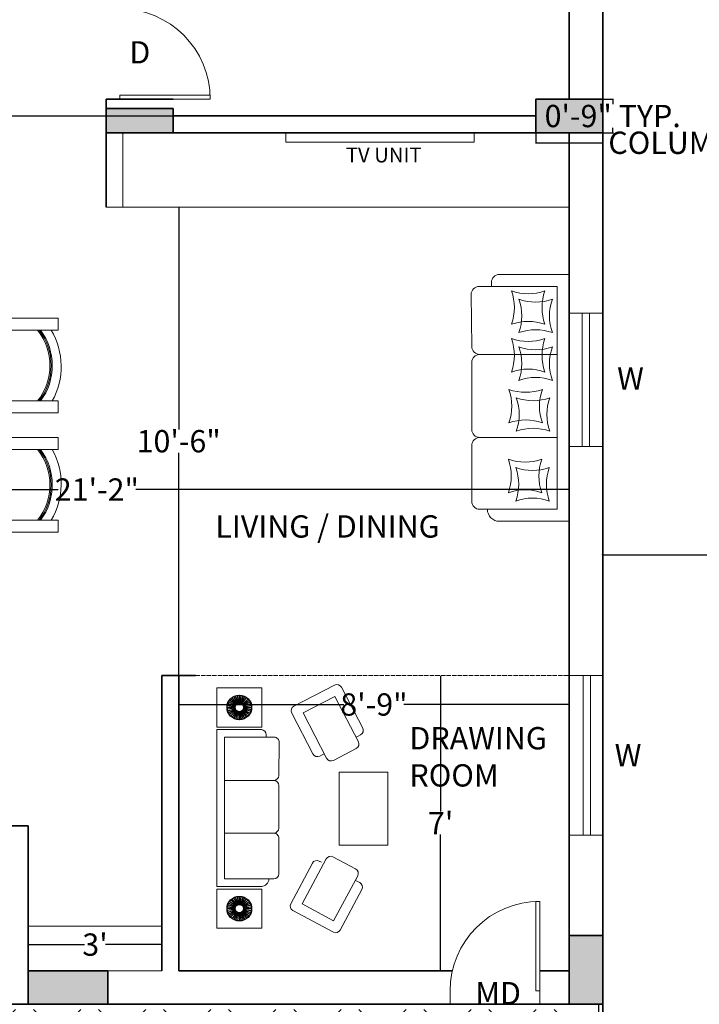
# Model space of a CAD drawing. Units: inches. Extents: x -2181 to 1225, y -80 to 4016.
# Tile 8 of 10: x 839 to 1021, y 191 to 456. Entities that reach past the tile are written whole.
import ezdxf

# ---------------------------------------------------------------- set-up
doc = ezdxf.new("R2010")
doc.units = ezdxf.units.IN
doc.header["$MEASUREMENT"] = 0
doc.linetypes.add('ACAD_ISO02W100', pattern=[15, 12, -3])
for name, color, linetype, lineweight in [('A-ANNO-DIMS', 2, 'Continuous', 18), ('A-ANNO-TEXT', 7, 'Continuous', 18), ('A-AREA-IDEN', 7, 'Continuous', 18), ('A-COLS', 7, 'Continuous', 35), ('A-COLS-PATT', 252, 'Continuous', 13), ('A-DOOR', 3, 'Continuous', 18), ('A-FLOR', 7, 'Continuous', 25), ('A-FLOR-PATT', 252, 'Continuous', 13), ('A-FURN', 30, 'Continuous', 18), ('A-GLAZ', 4, 'Continuous', 18), ('A-MILL', 8, 'Continuous', 18), ('A-WALL', 7, 'Continuous', 35), ('A-WALL-OVHD', 7, 'ACAD_ISO02W100', 18)]:
    doc.layers.add(name, color=color, linetype=linetype, lineweight=lineweight)
doc.layers.add('LAMP', color=2, linetype='Continuous')
doc.styles.get("Standard").update_dxf_attribs({"font": 'arial.ttf'})
doc.dimstyles.get("Standard").update_dxf_attribs({"dimtxt": 6, "dimasz": 0.18, "dimexe": 0.18, "dimexo": 0.0625, "dimgap": 0.09, "dimtad": 0, "dimtih": 1, "dimtoh": 1, "dimdec": 4, "dimzin": 0, "dimdsep": 46, "dimlunit": 4, "dimtxsty": 'Standard', "dimcen": 0.09, "dimadec": 0, "dimazin": 0, "dimtfac": 1, "dimtdec": 4, "dimtofl": 0, "dimtmove": 0, "dimatfit": 3, "dimfxl": 1, "dimtolj": 1, "dimtzin": 0, "dimarcsym": 0})

# ---------------------------------------------------------------- blocks, each defined once
blk = doc.blocks.new('*U2')
for p, q in [((0, 0), (0, -6)), ((40, 0), (40, -6))]:
    blk.add_line(p, q)
blk.add_lwpolyline([(0, 0), (0, 40), (1.75, 40), (1.75, 0)], close=True)
blk.add_arc((0, 0), 40, 0, 90)
blk = doc.blocks.new('*U18')
blk.add_line((3.3, 4.46), (3.3, 6.59))
for radius in [3.3, 1.16]:
    blk.add_circle((3.3, 3.3), radius)
blk = doc.blocks.new('*U17')
at = {"layer": 'LAMP', "transparency": 16777216}
for p, rotation in [((-44.82, 106.18), 44.99999999999992), ((-40.16, 110.84), 134.9999999999996), ((-44.82, 115.5), 224.9999999999994), ((-49.48, 110.84), 314.9999999999993), ((-45.55, 106.23), 35.99999999999994), ((-44.09, 106.23), 53.9999999999999), ((-40.22, 110.11), 125.9999999999997), ((-40.22, 111.57), 143.9999999999996), ((-44.09, 115.44), 215.9999999999994), ((-45.55, 115.44), 233.9999999999994), ((-49.43, 111.57), 305.9999999999992), ((-49.43, 110.11), 323.9999999999993), ((-46.26, 106.4), 26.99999999999998), ((-43.38, 106.4), 62.99999999999984), ((-40.39, 109.4), 116.9999999999997), ((-40.39, 112.28), 152.9999999999996), ((-43.38, 115.27), 206.9999999999994), ((-46.26, 115.27), 242.9999999999994), ((-49.26, 112.28), 296.9999999999993), ((-49.26, 109.4), 332.9999999999992), ((-46.94, 106.68), 17.99999999999997), ((-42.7, 106.68), 71.9999999999998), ((-40.67, 108.72), 107.9999999999997), ((-40.67, 112.96), 161.9999999999995), ((-42.7, 114.99), 197.9999999999995), ((-46.94, 114.99), 251.9999999999995), ((-48.98, 112.96), 287.9999999999994), ((-48.98, 108.72), 341.9999999999992), ((-47.56, 107.07), 8.999999999999984), ((-42.08, 107.07), 80.99999999999979), ((-41.05, 108.1), 98.99999999999974), ((-41.05, 113.58), 170.9999999999995), ((-42.08, 114.61), 188.9999999999995), ((-47.56, 114.61), 260.9999999999993), ((-48.59, 113.58), 278.9999999999992), ((-48.59, 108.1), 350.9999999999993), ((-41.52, 107.54), 89.99999999999976), ((-41.52, 114.14), 180), ((-48.12, 114.14), 269.9999999999993)]:
    blk.add_blockref('*U18', p, dxfattribs=dict(at, rotation=rotation))
blk.add_blockref('*U18', (-48.12, 107.54), dxfattribs=at)
blk = doc.blocks.new('*U15')
blk.add_line((3.3, 4.46), (3.3, 6.59))
for radius in [3.3, 1.16]:
    blk.add_circle((3.3, 3.3), radius)
blk = doc.blocks.new('*U16')
at = {"layer": 'LAMP', "transparency": 16777216}
for p, rotation in [((-44.82, 106.18), 44.99999999999992), ((-40.16, 110.84), 134.9999999999996), ((-44.82, 115.5), 224.9999999999994), ((-49.48, 110.84), 314.9999999999993), ((-45.55, 106.23), 35.99999999999994), ((-44.09, 106.23), 53.9999999999999), ((-40.22, 110.11), 125.9999999999997), ((-40.22, 111.57), 143.9999999999996), ((-44.09, 115.44), 215.9999999999994), ((-45.55, 115.44), 233.9999999999994), ((-49.43, 111.57), 305.9999999999992), ((-49.43, 110.11), 323.9999999999993), ((-46.26, 106.4), 26.99999999999998), ((-43.38, 106.4), 62.99999999999984), ((-40.39, 109.4), 116.9999999999997), ((-40.39, 112.28), 152.9999999999996), ((-43.38, 115.27), 206.9999999999994), ((-46.26, 115.27), 242.9999999999994), ((-49.26, 112.28), 296.9999999999993), ((-49.26, 109.4), 332.9999999999992), ((-46.94, 106.68), 17.99999999999997), ((-42.7, 106.68), 71.9999999999998), ((-40.67, 108.72), 107.9999999999997), ((-40.67, 112.96), 161.9999999999995), ((-42.7, 114.99), 197.9999999999995), ((-46.94, 114.99), 251.9999999999995), ((-48.98, 112.96), 287.9999999999994), ((-48.98, 108.72), 341.9999999999992), ((-47.56, 107.07), 8.999999999999984), ((-42.08, 107.07), 80.99999999999979), ((-41.05, 108.1), 98.99999999999974), ((-41.05, 113.58), 170.9999999999995), ((-42.08, 114.61), 188.9999999999995), ((-47.56, 114.61), 260.9999999999993), ((-48.59, 113.58), 278.9999999999992), ((-48.59, 108.1), 350.9999999999993), ((-41.52, 107.54), 89.99999999999976), ((-41.52, 114.14), 180), ((-48.12, 114.14), 269.9999999999993)]:
    blk.add_blockref('*U15', p, dxfattribs=dict(at, rotation=rotation))
blk.add_blockref('*U15', (-48.12, 107.54), dxfattribs=at)
blk = doc.blocks.new('*D25')
at = {"layer": 'A-ANNO-DIMS', "color": 0, "lineweight": -2, "transparency": 16777216}
for p, q in [((995.51, 312.49), (995.51, 312.61)), ((1087.01, 312.49), (1087.01, 312.61)), ((995.69, 312.43), (1031.04, 312.43)), ((1086.83, 312.43), (1051.49, 312.43))]:
    blk.add_line(p, q, dxfattribs=at)
at = {"layer": 'A-ANNO-DIMS', "color": 0, "transparency": 16777216}
for points in [[(995.69, 312.46), (995.69, 312.4), (995.51, 312.43)], [(1086.83, 312.46), (1086.83, 312.4), (1087.01, 312.43)]]:
    blk.add_solid(points, dxfattribs=at)
at = {"layer": 'Defpoints', "color": 0, "transparency": 16777216}
for p in [(995.51, 312.43), (1087.01, 312.43), (1087.01, 312.43)]:
    blk.add_point(p, dxfattribs=at)
at = {"layer": 'A-ANNO-DIMS', "color": 0, "transparency": 16777216, "insert": (1041.26, 312.43), "char_height": 6, "attachment_point": 5}
blk.add_mtext('\\A1;7\'-7{\\H1x;\\S1/2;}"', dxfattribs=at)
blk = doc.blocks.new('*D53')
at = {"layer": 'A-ANNO-DIMS', "color": 0, "lineweight": -2, "transparency": 16777216}
for p, q in [((881.51, 279.92), (881.51, 271.97)), ((986.51, 279.92), (986.51, 271.97)), ((881.69, 272.15), (925.95, 272.15)), ((986.33, 272.15), (942.08, 272.15))]:
    blk.add_line(p, q, dxfattribs=at)
at = {"layer": 'A-ANNO-DIMS', "color": 0, "transparency": 16777216}
for points in [[(881.69, 272.18), (881.69, 272.12), (881.51, 272.15)], [(986.33, 272.18), (986.33, 272.12), (986.51, 272.15)]]:
    blk.add_solid(points, dxfattribs=at)
at = {"layer": 'Defpoints', "color": 0, "transparency": 16777216}
for p in [(881.51, 279.98), (986.51, 279.98), (986.51, 272.15)]:
    blk.add_point(p, dxfattribs=at)
at = {"layer": 'A-ANNO-DIMS', "color": 0, "transparency": 16777216, "insert": (934.01, 272.15), "char_height": 6, "attachment_point": 5}
blk.add_mtext('\\A1;8\'-9"', dxfattribs=at)
blk = doc.blocks.new('*D54')
at = {"layer": 'A-ANNO-DIMS', "color": 0, "lineweight": -2, "transparency": 16777216}
for p, q in [((951.95, 279.8), (951.95, 243.32)), ((952.01, 279.98), (952.13, 279.98)), ((951.95, 200.66), (951.95, 237.14)), ((955.06, 200.48), (951.77, 200.48))]:
    blk.add_line(p, q, dxfattribs=at)
at = {"layer": 'A-ANNO-DIMS', "color": 0, "transparency": 16777216}
for points in [[(951.92, 279.8), (951.98, 279.8), (951.95, 279.98)], [(951.92, 200.66), (951.98, 200.66), (951.95, 200.48)]]:
    blk.add_solid(points, dxfattribs=at)
at = {"layer": 'Defpoints', "color": 0, "transparency": 16777216}
for p in [(951.95, 279.98), (951.95, 279.98), (955.12, 200.48)]:
    blk.add_point(p, dxfattribs=at)
at = {"layer": 'A-ANNO-DIMS', "color": 0, "transparency": 16777216, "insert": (951.95, 240.23), "char_height": 6, "attachment_point": 5}
blk.add_mtext("\\A1;7'", dxfattribs=at)
blk = doc.blocks.new('*D55')
at = {"layer": 'A-ANNO-DIMS', "color": 0, "lineweight": -2, "transparency": 16777216}
for p, q in [((841.01, 212.42), (841.01, 207.37)), ((877.01, 212.42), (877.01, 207.37)), ((841.19, 207.55), (856.17, 207.55)), ((876.83, 207.55), (861.86, 207.55))]:
    blk.add_line(p, q, dxfattribs=at)
at = {"layer": 'A-ANNO-DIMS', "color": 0, "transparency": 16777216}
for points in [[(841.19, 207.58), (841.19, 207.52), (841.01, 207.55)], [(876.83, 207.58), (876.83, 207.52), (877.01, 207.55)]]:
    blk.add_solid(points, dxfattribs=at)
at = {"layer": 'Defpoints', "color": 0, "transparency": 16777216}
for p in [(841.01, 212.48), (877.01, 212.48), (877.01, 207.55)]:
    blk.add_point(p, dxfattribs=at)
at = {"layer": 'A-ANNO-DIMS', "color": 0, "transparency": 16777216, "insert": (859.01, 207.55), "char_height": 6, "attachment_point": 5}
blk.add_mtext("\\A1;3'", dxfattribs=at)
blk = doc.blocks.new('*D57')
at = {"layer": 'A-ANNO-DIMS', "color": 0, "lineweight": -2, "transparency": 16777216}
for p, q in [((732.51, 330.05), (732.51, 330.16)), ((732.69, 329.98), (849.07, 329.98)), ((986.33, 329.98), (869.96, 329.98)), ((986.51, 330.05), (986.51, 330.16))]:
    blk.add_line(p, q, dxfattribs=at)
at = {"layer": 'A-ANNO-DIMS', "color": 0, "transparency": 16777216}
for points in [[(732.69, 330.01), (732.69, 329.95), (732.51, 329.98)], [(986.33, 330.01), (986.33, 329.95), (986.51, 329.98)]]:
    blk.add_solid(points, dxfattribs=at)
at = {"layer": 'Defpoints', "color": 0, "transparency": 16777216}
for p in [(732.51, 329.98), (986.51, 329.98), (986.51, 329.98)]:
    blk.add_point(p, dxfattribs=at)
at = {"layer": 'A-ANNO-DIMS', "color": 0, "transparency": 16777216, "insert": (859.51, 329.98), "char_height": 6, "attachment_point": 5}
blk.add_mtext('\\A1;21\'-2"', dxfattribs=at)
blk = doc.blocks.new('*D58')
at = {"layer": 'A-ANNO-DIMS', "color": 0, "lineweight": -2, "transparency": 16777216}
for p, q in [((881.51, 405.8), (881.51, 346.14)), ((881.58, 405.98), (881.69, 405.98)), ((881.51, 280.16), (881.51, 339.83)), ((881.58, 279.98), (881.69, 279.98))]:
    blk.add_line(p, q, dxfattribs=at)
at = {"layer": 'A-ANNO-DIMS', "color": 0, "transparency": 16777216}
for points in [[(881.48, 405.8), (881.54, 405.8), (881.51, 405.98)], [(881.48, 280.16), (881.54, 280.16), (881.51, 279.98)]]:
    blk.add_solid(points, dxfattribs=at)
at = {"layer": 'Defpoints', "color": 0, "transparency": 16777216}
for p in [(881.51, 405.98), (881.51, 405.98), (881.51, 279.98)]:
    blk.add_point(p, dxfattribs=at)
at = {"layer": 'A-ANNO-DIMS', "color": 0, "transparency": 16777216, "insert": (881.51, 342.98), "char_height": 6, "attachment_point": 5}
blk.add_mtext('\\A1;10\'-6"', dxfattribs=at)
blk = doc.blocks.new('DINING-CHAIR-SIDE')
for p, q in [((0.79, 22.26), (0.79, 25.47)), ((19.33, 22.26), (19.33, 25.47)), ((0.79, 0), (0.79, 3.21)), ((19.33, 3.21), (19.33, 0))]:
    blk.add_line(p, q)
for points in [[(0.79, 25.47), (19.33, 25.47)], [(0.79, 22.26), (22.53, 22.26), (22.53, 3.21), (0.79, 3.21)], [(19.33, 0), (0.79, 0)]]:
    blk.add_lwpolyline(points)
for centre, radius, start, end in [((19.12, 12.45), 19.13, 149.1418, 208.8973), ((18.29, 12.73), 15.92, 143.2428, 216.7572), ((18.29, 12.73), 15.6, 142.3578, 217.6422), ((18.29, 12.73), 15.28, 141.4242, 218.5758)]:
    blk.add_arc(centre, radius, start, end)
blk = doc.blocks.new('COL-18X9')
blk.add_lwpolyline([(0, 9), (18, 9), (18, 0), (0, 0)], close=True)
blk = doc.blocks.new('*D98')
at = {"layer": 'A-ANNO-DIMS', "color": 0, "lineweight": -2, "transparency": 16777216}
for p, q in [((977.51, 425.92), (977.51, 423.1)), ((995.51, 425.92), (995.51, 423.1)), ((977.69, 423.28), (995.33, 423.28)), ((995.51, 423.28), (995.69, 423.28))]:
    blk.add_line(p, q, dxfattribs=at)
at = {"layer": 'A-ANNO-DIMS', "color": 0, "transparency": 16777216}
for points in [[(977.69, 423.31), (977.69, 423.25), (977.51, 423.28)], [(995.33, 423.31), (995.33, 423.25), (995.51, 423.28)]]:
    blk.add_solid(points, dxfattribs=at)
at = {"layer": 'Defpoints', "color": 0, "transparency": 16777216}
for p in [(977.51, 425.98), (995.51, 425.98), (995.51, 423.28)]:
    blk.add_point(p, dxfattribs=at)
at = {"layer": 'A-ANNO-DIMS', "color": 0, "transparency": 16777216, "insert": (1033.36, 423.28), "char_height": 6, "attachment_point": 5}
blk.add_mtext('\\A1;COLUMN 1\'-6" TYP.', dxfattribs=at)
blk = doc.blocks.new('*D99')
at = {"layer": 'A-ANNO-DIMS', "color": 0, "lineweight": -2, "transparency": 16777216}
for p, q in [((995.58, 434.98), (998.39, 434.98)), ((998.21, 434.8), (998.21, 433.64)), ((998.21, 426.16), (998.21, 427.33)), ((995.58, 425.98), (998.39, 425.98))]:
    blk.add_line(p, q, dxfattribs=at)
at = {"layer": 'A-ANNO-DIMS', "color": 0, "transparency": 16777216}
for points in [[(998.18, 434.8), (998.24, 434.8), (998.21, 434.98)], [(998.18, 426.16), (998.24, 426.16), (998.21, 425.98)]]:
    blk.add_solid(points, dxfattribs=at)
at = {"layer": 'Defpoints', "color": 0, "transparency": 16777216}
for p in [(995.51, 434.98), (998.21, 434.98), (995.51, 425.98)]:
    blk.add_point(p, dxfattribs=at)
at = {"layer": 'A-ANNO-DIMS', "color": 0, "transparency": 16777216, "insert": (998.21, 430.48), "char_height": 6, "attachment_point": 5}
blk.add_mtext('\\A1;0\'-9" TYP.', dxfattribs=at)
blk = doc.blocks.new('*D131')
at = {"layer": 'A-ANNO-DIMS', "color": 0, "lineweight": -2, "transparency": 16777216}
for p, q in [((976.64, 563.98), (-59.44, 563.98)), ((-59.26, 563.8), (-59.26, 500.43)), ((-59.26, 430.66), (-59.26, 494.04)), ((977.45, 430.48), (-59.44, 430.48))]:
    blk.add_line(p, q, dxfattribs=at)
at = {"layer": 'A-ANNO-DIMS', "color": 0, "transparency": 16777216}
for points in [[(-59.29, 563.8), (-59.23, 563.8), (-59.26, 563.98)], [(-59.29, 430.66), (-59.23, 430.66), (-59.26, 430.48)]]:
    blk.add_solid(points, dxfattribs=at)
at = {"layer": 'Defpoints', "color": 0, "transparency": 16777216}
for p in [(976.7, 563.98), (-59.26, 430.48), (977.51, 430.48)]:
    blk.add_point(p, dxfattribs=at)
at = {"layer": 'A-ANNO-DIMS', "color": 0, "transparency": 16777216, "insert": (-59.26, 497.23), "char_height": 6, "attachment_point": 5}
blk.add_mtext('\\A1;11\'-1 1/2"', dxfattribs=at)

msp = doc.modelspace()

# ---------------------------------------------------------------- hatches: boundary and pattern name
at = {"layer": 'A-COLS-PATT'}
h = msp.add_hatch(color=256, dxfattribs=at)
h.dxf.hatch_style = 1
h.paths.add_polyline_path([(995.51461, 209.98479), (986.51461, 209.98479), (986.51461, 191.48479), (995.51461, 191.48479)])
h.paths.add_polyline_path([(862.50488, 191.48479), (862.50488, 200.48479), (841.01461, 200.48479), (841.01461, 191.48479)])
h.paths.add_polyline_path([(995.51461, 425.98479), (995.51461, 434.98479), (977.51461, 434.98479), (977.51461, 425.98479)])
h.paths.add_polyline_path([(880.01461, 425.98479), (880.01461, 432.54138), (862.01461, 432.54138), (862.01461, 425.98479)])
h.paths.add_polyline_path([(880.82546, 563.98479), (880.82546, 572.98479), (862.01461, 572.98479), (862.01461, 563.98479)])
h.paths.add_polyline_path([(995.51461, 563.98479), (995.51461, 572.98479), (976.70377, 572.98479), (976.70377, 563.98479)])
h.paths.add_polyline_path([(674.51461, 572.98479), (665.51461, 572.98479), (665.51461, 556.48479), (674.51461, 556.48479)])
h.paths.add_polyline_path([(674.51461, 442.48479), (665.51461, 442.48479), (665.51461, 425.98479), (674.51461, 425.98479)])
at = {"layer": 'A-FLOR-PATT'}
h = msp.add_hatch(dxfattribs=at)
h.set_pattern_fill('ANGLE', color=256, scale=45, angle=45)
h.set_pattern_definition([(45, (0, 0), (-8.75045, 8.75045), [9, -3.375]), (135, (0, 0), (-8.75045, -8.75045), [9, -3.375])])
h.paths.add_polyline_path([(665.51461, 191.48479), (665.51461, 136.48479), (674.51461, 136.48479), (674.51461, 137.48479), (994.51461, 137.48479), (994.51461, 191.48479)])

# ---------------------------------------------------------------- linework, layer by layer
at = {"layer": 'A-COLS'}
for p, q in [((977.51461, 434.98479), (995.51461, 434.98479)), ((880.01461, 432.54138), (862.01461, 432.54138)), ((986.51461, 425.98479), (995.51461, 425.98479))]:
    msp.add_line(p, q, dxfattribs=at)
for points in [[(880.01461, 432.54138), (880.01461, 425.98479), (862.01461, 425.98479), (862.01461, 434.98479), (880.01461, 434.98479)], [(977.51461, 425.98479), (977.51461, 434.98479)], [(986.51461, 209.98479), (995.51461, 209.98479)]]:
    msp.add_lwpolyline(points, dxfattribs=at)
msp.add_lwpolyline([(841.01461, 200.48479), (862.50488, 200.48479), (862.50488, 191.48479), (841.01461, 191.48479)], close=True, dxfattribs=at)
at = {"layer": 'A-FLOR'}
msp.add_lwpolyline([(994.51461, 137.48479), (994.51461, 191.48479)], dxfattribs=at)
at = {"layer": 'A-FURN'}
for p, q in [((983.28882, 366.34519), (962.47646, 366.34519)), ((961.4012, 344.01286), (961.4012, 344.01067)), ((983.28882, 344.00116), (962.4774, 344.01021)), ((920.66303, 258.90305), (919.75396, 258.42993)), ((893.8348, 251.72826), (907.05875, 251.72826)), ((893.8348, 237.5311), (907.05816, 237.53685)), ((907.74196, 237.53853), (907.74196, 237.53714))]:
    msp.add_line(p, q, dxfattribs=at)
for points in [[(986.51461, 321.4323), (986.51461, 387.85049), (967.75164, 387.85049, 0.414213562), (965.60111, 385.69996), (965.60111, 384.62469)], [(983.28882, 324.6581), (983.28882, 384.62469), (962.30166, 384.62469, 0.417877186), (960.1513, 382.4473), (960.32593, 368.46885, 0.410559405), (962.47629, 366.34519), (983.28882, 366.34519)], [(960.32593, 364.19466), (960.32593, 346.16339, 0.414213562), (962.47646, 344.01286), (983.28882, 344.01286)], [(960.32593, 341.85968), (960.32593, 326.80862, 0.414213562), (962.47646, 324.6581), (983.28882, 324.6581)], [(964.52584, 324.6581), (964.52584, 324.6581, 0.414213562), (967.75164, 321.4323), (986.51461, 321.4323)], [(920.05698, 258.58764), (919.45094, 258.27222, -0.414213562), (917.60802, 258.85348), (911.9007, 269.81962, -0.414213562), (912.48196, 271.66254), (923.43749, 277.36434, -0.414213562), (925.28041, 276.78308), (930.98773, 265.81695, -0.414213562), (930.40647, 263.97402), (929.80042, 263.65861), (929.19438, 263.34319)], [(891.78516, 223.19108), (891.78516, 265.3925), (903.70696, 265.3925, -0.414213562), (905.07338, 264.02608), (905.07338, 263.34287)], [(893.8348, 225.24072), (893.8348, 263.34287), (907.16982, 263.34287, -0.417877186), (908.53613, 261.95937), (908.42518, 253.07762, -0.410559405), (907.05886, 251.72826), (893.8348, 251.72826)], [(908.42518, 250.36184), (908.42518, 238.90496, -0.414213562), (907.05875, 237.53853), (893.8348, 237.53853)], [(908.42518, 236.17042), (908.42518, 226.60714, -0.414213562), (907.05875, 225.24072), (893.8348, 225.24072)], [(919.90911, 229.70718), (919.30633, 230.02879, 0.414213562), (917.45755, 229.46643), (911.63823, 218.55932, 0.414213562), (912.20059, 216.71054), (923.09715, 210.89685, 0.414213562), (924.94593, 211.4592), (930.76525, 222.36632, 0.414213562), (930.20289, 224.2151), (929.60011, 224.53671), (928.99733, 224.85831)], [(905.75659, 225.24072), (905.75659, 225.24072, -0.414213562), (903.70696, 223.19108), (891.78516, 223.19108)]]:
    msp.add_lwpolyline(points, format="xyb", dxfattribs=at)
for points in [[(967.75164, 387.85049), (967.51697, 387.85049)], [(967.51697, 321.4323), (967.75164, 321.4323)], [(891.78516, 276.64518), (891.78516, 266.07571)], [(903.85606, 276.64518), (891.78516, 276.64518)], [(891.78516, 276.64518), (891.78516, 266.07571)], [(903.85606, 276.64518), (891.78516, 276.64518)], [(903.85606, 266.07571), (903.85606, 276.64518)], [(903.85606, 266.07571), (903.85606, 276.64518)], [(891.78516, 266.07571), (903.85606, 266.07571)], [(891.78516, 266.07571), (903.85606, 266.07571)], [(903.70696, 265.3925), (903.85606, 265.3925)], [(903.85606, 223.19108), (903.70696, 223.19108)], [(891.78516, 222.50787), (891.78516, 211.93841)], [(903.85606, 222.50787), (891.78516, 222.50787)], [(891.78516, 222.50787), (891.78516, 211.93841)], [(903.85606, 222.50787), (891.78516, 222.50787)], [(891.78516, 222.50787), (891.78516, 211.93841)], [(903.85606, 222.50787), (891.78516, 222.50787)], [(903.85606, 211.93841), (903.85606, 222.50787)], [(903.85606, 211.93841), (903.85606, 222.50787)], [(903.85606, 211.93841), (903.85606, 222.50787)], [(891.78516, 211.93841), (903.85606, 211.93841)], [(891.78516, 211.93841), (903.85606, 211.93841)], [(891.78516, 211.93841), (903.85606, 211.93841)]]:
    msp.add_lwpolyline(points, dxfattribs=at)
for points in [[(921.29386, 257.69096), (914.95571, 269.86919), (923.48706, 274.30933), (929.82521, 262.1311, -0.414213562), (929.24395, 260.28817), (923.13679, 257.1097, -0.414213562)], [(921.1551, 230.59115), (914.69258, 218.47846), (923.17801, 213.9512), (929.64054, 226.06388, 0.414213562), (929.07818, 227.91266), (923.00388, 231.1535, 0.414213562)]]:
    msp.add_lwpolyline(points, format="xyb", close=True, dxfattribs=at)
msp.add_lwpolyline([(924.68117, 253.97634), (937.72776, 253.97634), (937.72776, 234.27037), (924.68117, 234.27037)], close=True, dxfattribs=at)
for centre, radius, start, end in [((975.48814, 395.98818), 13.32748, 250.2663432, 289.7336568), ((958.44335, 378.94339), 13.32748, 340.2663432, 19.7336568), ((992.53293, 378.94339), 13.32748, 160.2663432, 199.7336568), ((977.48811, 393.74472), 13.32748, 250.2663432, 289.7336568), ((960.44332, 376.69994), 13.32748, 340.2663432, 19.7336568), ((994.53289, 376.69994), 13.32748, 160.2663432, 199.7336568), ((975.48814, 361.8986), 13.32748, 70.2663432, 109.7336568), ((977.48811, 359.65515), 13.32748, 70.2663432, 109.7336568), ((975.48814, 383.14097), 13.32748, 250.2663432, 289.7336568), ((958.44335, 366.09619), 13.32748, 340.2663432, 19.7336568), ((977.48811, 380.89752), 13.32748, 250.2663432, 289.7336568), ((960.44332, 363.85273), 13.32748, 340.2663432, 19.7336568), ((992.53293, 366.09619), 13.32748, 160.2663432, 199.7336568), ((994.53289, 363.85273), 13.32748, 160.2663432, 199.7336568), ((962.47646, 364.19466), 2.15053, 90, 180), ((975.48814, 349.0514), 13.32748, 70.2663432, 109.7336568), ((977.48811, 346.80795), 13.32748, 70.2663432, 109.7336568), ((974.79693, 369.46492), 13.32748, 250.2663432, 289.7336568), ((957.75215, 352.42014), 13.32748, 340.2663432, 19.7336568), ((991.84172, 352.42014), 13.32748, 160.2663432, 199.7336568), ((976.7969, 367.22147), 13.32748, 250.2663432, 289.7336568), ((959.75211, 350.17668), 13.32748, 340.2663432, 19.7336568), ((993.84169, 350.17668), 13.32748, 160.2663432, 199.7336568), ((974.79693, 335.37535), 13.32748, 70.2663432, 109.7336568), ((976.7969, 333.1319), 13.32748, 70.2663432, 109.7336568), ((962.47646, 341.85968), 2.15053, 89.9751027, 180), ((974.65869, 350.67762), 13.32748, 250.2663432, 289.7336568), ((957.6139, 333.63283), 13.32748, 340.2663432, 19.7336568), ((991.70348, 333.63283), 13.32748, 160.2663432, 199.7336568), ((976.65866, 348.43417), 13.32748, 250.2663432, 289.7336568), ((959.61387, 331.38938), 13.32748, 340.2663432, 19.7336568), ((993.70345, 331.38938), 13.32748, 160.2663432, 199.7336568), ((974.65869, 316.58805), 13.32748, 70.2663432, 109.7336568), ((976.65866, 314.34459), 13.32748, 70.2663432, 109.7336568), ((907.05875, 250.36184), 1.36642, 360, 450), ((907.05875, 236.17042), 1.36642, 360, 450.0248973)]:
    msp.add_arc(centre, radius, start, end, dxfattribs=at)
at = {"layer": 'A-GLAZ'}
for p, q in [((986.51461, 377.43623), (995.51461, 377.43623)), ((990.01461, 341.51785), (990.01461, 377.43623)), ((992.01461, 341.51785), (992.01461, 377.43623)), ((986.51461, 341.51785), (995.51461, 341.51785)), ((986.51461, 279.98479), (995.51461, 279.98479)), ((990.25268, 279.98479), (990.25268, 236.98479)), ((992.25268, 279.98479), (992.25268, 236.98479))]:
    msp.add_line(p, q, dxfattribs=at)
msp.add_lwpolyline([(986.51461, 236.98479), (995.51461, 236.98479)], dxfattribs=at)
at = {"layer": 'A-MILL'}
for points in [[(866.51461, 405.98479), (866.51461, 425.98479)], [(862.01461, 405.98479), (986.51461, 405.98479)], [(841.01461, 212.48479), (877.01461, 212.48479)], [(841.01461, 200.48479), (877.01461, 200.48479)]]:
    msp.add_lwpolyline(points, dxfattribs=at)
msp.add_lwpolyline([(910.31091, 425.98479), (960.93988, 425.98479), (960.93988, 423.467), (910.31091, 423.467)], close=True, dxfattribs=at)
at = {"layer": 'A-WALL'}
for p, q in [((886.01461, 279.98479), (877.01461, 279.98479)), ((836.51461, 239.48479), (841.01461, 239.48479))]:
    msp.add_line(p, q, dxfattribs=at)
for points in [[(995.51461, 136.48479), (995.51461, 572.98479), (665.51461, 572.98479)], [(986.51461, 434.98479), (986.51461, 563.98479)], [(862.01461, 405.98479), (862.01461, 434.98479)], [(977.51461, 430.48479), (880.01461, 430.48479)], [(986.51461, 425.98479), (866.51461, 425.98479)], [(986.51461, 191.48479), (986.51461, 425.98479)], [(877.01461, 200.48479), (877.01461, 279.98479)], [(881.51461, 200.48479), (881.51461, 279.98479)], [(841.01461, 191.48479), (841.01461, 239.48479)], [(881.51461, 200.48479), (955.12217, 200.48479)], [(978.59298, 200.48479), (986.51461, 200.48479)], [(665.51461, 191.48479), (995.51461, 191.48479)]]:
    msp.add_lwpolyline(points, dxfattribs=at)
at = {"layer": 'A-WALL-OVHD', "ltscale": 0.1}
msp.add_lwpolyline([(886.01461, 279.98479), (986.51461, 279.98479)], dxfattribs=at)

# ---------------------------------------------------------------- block references
at = {"layer": 'A-COLS'}
msp.add_blockref('COL-18X9', (977.515, 425.985), dxfattribs=at)
at = {"layer": 'A-DOOR', "extrusion": (0, 0, -1), "xscale": 0.608774911433326, "yscale": 0.608774911433326, "zscale": -0.608774911433326, "rotation": 90.00000000000003}
msp.add_blockref('*U2', (-865.66726, 434.98479), dxfattribs=at)
at = {"layer": 'A-DOOR', "extrusion": (0, 0, -1), "xscale": 0.6020316206523724, "yscale": 0.6020316206523724, "zscale": -0.6020316206523724}
msp.add_blockref('*U2', (-978.59298, 195.09698), dxfattribs=at)
at = {"layer": 'A-FURN', "extrusion": (0, 0, -1), "zscale": -1}
msp.add_blockref('DINING-CHAIR-SIDE', (-849.90472, 350.605), dxfattribs=at)
at = {"layer": 'A-FURN', "rotation": 180}
msp.add_blockref('DINING-CHAIR-SIDE', (849.90472, 343.96907), dxfattribs=at)
at = {"layer": 'LAMP'}
for name, p in [('*U17', (942.64185, 160.52128)), ('*U16', (942.64185, 106.38397))]:
    msp.add_blockref(name, p, dxfattribs=at)

# ---------------------------------------------------------------- texts
at = {"layer": 'A-ANNO-TEXT', "attachment_point": 1}
for s, width, insert, char_height in [('D', 291.4178321, (868.25204, 450.61664), 6), ('TV UNIT ', 53.2864443, (926.45246, 421.99761), 4), ('W', 291.4178321, (999.40302, 362.89363), 6), ('W', 291.4178321, (998.74819, 261.48777), 6), ('MD', 291.4178321, (961.25385, 197.48479), 6)]:
    msp.add_mtext_dynamic_manual_height_columns(s, width=width, gutter_width=1, heights=[0], dxfattribs=dict(at, insert=insert, char_height=char_height))
at = {"layer": 'A-AREA-IDEN', "char_height": 6, "attachment_point": 1}
for s, insert in [('LIVING / DINING', (891.38663, 323.05205)), ('DRAWING \\PROOM', (943.55112, 266.07613))]:
    msp.add_mtext_dynamic_manual_height_columns(s, width=291.4178321, gutter_width=1, heights=[0], dxfattribs=dict(at, insert=insert))

# ---------------------------------------------------------------- dimensions: what is measured, and where the dimension line sits
at = {"layer": 'A-ANNO-DIMS'}
for base, p1, p2, override, picture, middle in [((-59.2566, 430.48478), (976.70377, 563.98478), (977.51461, 430.48478), {"dimdec": 1, "dimlfac": 1, "dimrnd": 0, "dimzin": 1, "dimdsep": 46, "dimlunit": 4, "dimfrac": 2}, '*D131', (-59.2566, 497.23478)), ((881.51461, 405.98479), (881.51461, 279.98479), (881.51461, 405.98479), {"dimclrd": 0, "dimclre": 0, "dimclrt": 0}, '*D58', (881.51461, 342.98479))]:
    dim = msp.add_linear_dim(base=base, p1=p1, p2=p2, angle=90, dimstyle='Standard', override=override, dxfattribs=at)
    dim.commit()
    dim.dimension.update_dxf_attribs({"geometry": picture, "text_midpoint": middle})
dim = msp.add_linear_dim(base=(995.51461, 423.28479), p1=(977.51461, 425.98479), p2=(995.51461, 425.98479), text='COLUMN <> TYP.', dimstyle='Standard', override={"dimdec": 1, "dimlfac": 1, "dimrnd": 0, "dimzin": 1, "dimdsep": 46, "dimlunit": 4, "dimfrac": 2}, dxfattribs=at)
dim.commit()
dim.dimension.update_dxf_attribs({"geometry": '*D98', "text_midpoint": (1033.36238, 423.28479)})
for base, p1, p2, text, override, picture, middle in [((998.21461, 434.98479), (995.51461, 425.98479), (995.51461, 434.98479), '<> TYP.', {"dimdec": 1, "dimlfac": 1, "dimrnd": 0, "dimzin": 1, "dimdsep": 46, "dimlunit": 4, "dimfrac": 2}, '*D99', (998.21461, 430.48479)), ((951.94755, 279.98479), (955.12217, 200.48479), (951.94755, 279.98479), "7'", {"dimclrd": 0, "dimclre": 0, "dimclrt": 0}, '*D54', (951.94755, 240.23479))]:
    dim = msp.add_linear_dim(base=base, p1=p1, p2=p2, angle=90, text=text, dimstyle='Standard', override=override, dxfattribs=at)
    dim.commit()
    dim.dimension.update_dxf_attribs({"geometry": picture, "text_midpoint": middle})
for base, p1, p2, picture, middle in [((986.51461, 329.98479), (732.51461, 329.98479), (986.51461, 329.98479), '*D57', (859.51461, 329.98479)), ((1087.01461, 312.43008), (995.51461, 312.43008), (1087.01461, 312.43008), '*D25', (1041.26461, 312.43008)), ((986.51461, 272.15252), (881.51461, 279.98479), (986.51461, 279.98479), '*D53', (934.01461, 272.15252)), ((877.01461, 207.55241), (841.01461, 212.48479), (877.01461, 212.48479), '*D55', (859.01461, 207.55241))]:
    dim = msp.add_linear_dim(base=base, p1=p1, p2=p2, dimstyle='Standard', override={"dimclrd": 0, "dimclre": 0, "dimclrt": 0}, dxfattribs=at)
    dim.commit()
    dim.dimension.update_dxf_attribs({"geometry": picture, "text_midpoint": middle})

doc.saveas('drawing.dxf')
